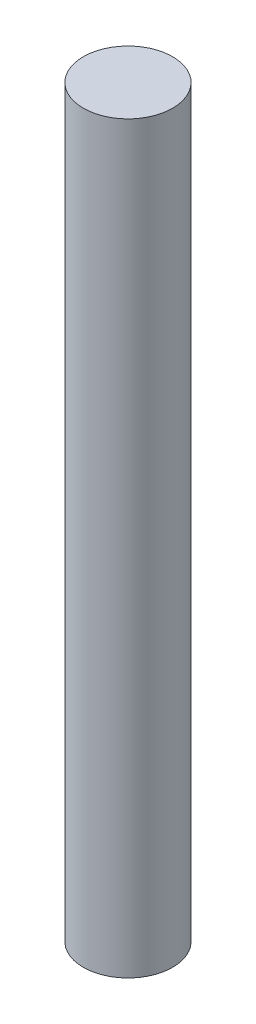
from build123d import *

# Parameters (mm, degrees)
SHAFT_PROFILE_24_R   = 12
SHAFT_24_X_200_DEPTH = 200


with BuildPart() as part:
    # Shaft Profile Ø24 → Shaft Ø24 x 200 (new body)
    with BuildSketch(Plane(origin=(0, 0, 0), x_dir=(1, 0, 0), z_dir=(0, 1, 0))):
        with Locations(Location((0, 0, 0), (0, 0, 270))):
            Circle(SHAFT_PROFILE_24_R)
    extrude(amount=SHAFT_24_X_200_DEPTH)


solid = part.part
